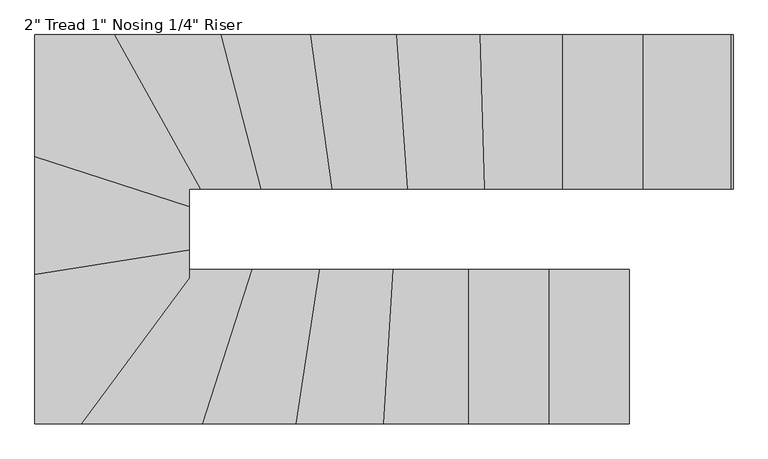
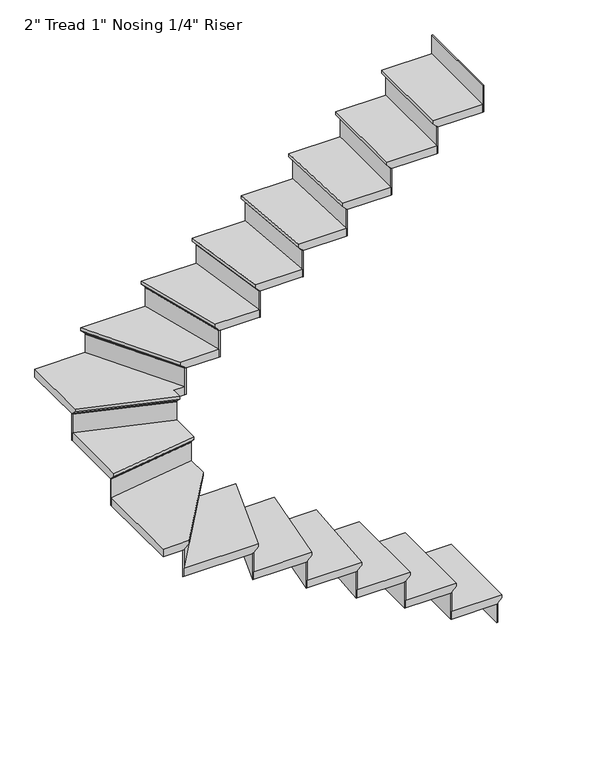
"""IFC4 building model written with IfcOpenShell, lengths in millimetres: stair flight geometry."""

from ifc_helpers import new_model, si_unit, origin, place, context, project, spatial, faceted_brep, source, transform, mapped, element, save


def stair_flight_959e1ed9(model_context):
    return source(origin(), model_context, "Body", "Brep", [
        faceted_brep([(-264.8831579, 264.4433073, 3350.6833333), (-264.8831579, 264.4433073, 3369.7333333), (-264.8831579, -271.8029286, 3369.7333333), (-264.8831579, -271.8029286, 3350.6833333), (-290.2831579, 264.4433073, 3325.2833333), (-290.2831579, -271.8029286, 3325.2833333), (-569.6831579, 264.4433073, 3369.7333333), (-569.6831579, -271.8029286, 3369.7333333), (-290.2831579, -271.8029286, 3318.9333333), (-569.6831579, -271.8029286, 3318.9333333), (-569.6831579, 264.4433073, 3318.9333333), (-290.2831579, 264.4433073, 3318.9333333)], [[[0, 1, 2, 3]], [[4, 0, 3, 5]], [[2, 1, 6, 7]], [[8, 9, 10, 11]], [[2, 7, 9, 8, 5, 3]], [[8, 11, 4, 5]], [[6, 1, 0, 4, 11, 10]], [[7, 6, 10, 9]]]),
        faceted_brep([(-290.2831579, 264.4433073, 3318.9333333), (-290.2831579, 264.4433073, 3200.4), (-296.6331579, 264.4433073, 3200.4), (-296.6331579, 264.4433073, 3318.9333333), (-290.2831579, -271.8029286, 3318.9333333), (-296.6331579, -271.8029286, 3318.9333333), (-296.6331579, -271.8029286, 3200.4), (-290.2831579, -271.8029286, 3200.4)], [[[0, 1, 2, 3]], [[4, 5, 6, 7]], [[1, 0, 4, 7]], [[2, 1, 7, 6]], [[3, 2, 6, 5]], [[0, 3, 5, 4]]]),
        faceted_brep([(-569.6831579, 264.4433073, 3488.2666667), (-569.6831579, 264.4433073, 3318.9333333), (-576.0331579, 264.4433073, 3318.9333333), (-576.0331579, 264.4433073, 3488.2666667), (-569.6831579, -271.8029286, 3488.2666667), (-576.0331579, -271.8029286, 3488.2666667), (-576.0331579, -271.8029286, 3318.9333333), (-569.6831579, -271.8029286, 3318.9333333)], [[[0, 1, 2, 3]], [[4, 5, 6, 7]], [[1, 0, 4, 7]], [[2, 1, 7, 6]], [[3, 2, 6, 5]], [[0, 3, 5, 4]]]),
        faceted_brep([(-544.2831579, -271.8029286, 3539.0666667), (-544.2831579, 264.4433073, 3539.0666667), (-849.0831579, 264.4433073, 3539.0666667), (-849.0831579, -271.8029286, 3539.0666667), (-569.6831579, -271.8029286, 3488.2666667), (-849.0831579, -271.8029286, 3488.2666667), (-849.0831579, 264.4433073, 3488.2666667), (-569.6831579, 264.4433073, 3488.2666667), (-569.6831579, -271.8029286, 3494.6166667), (-544.2831579, -271.8029286, 3520.0166667), (-569.6831579, 264.4433073, 3494.6166667), (-544.2831579, 264.4433073, 3520.0166667)], [[[0, 1, 2, 3]], [[4, 5, 6, 7]], [[0, 3, 5, 4, 8, 9]], [[4, 7, 10, 8]], [[2, 1, 11, 10, 7, 6]], [[3, 2, 6, 5]], [[11, 1, 0, 9]], [[10, 11, 9, 8]]]),
        faceted_brep([(-849.0831579, 264.4433073, 3657.6), (-849.0831579, 264.4433073, 3488.2666667), (-855.4331579, 264.4433073, 3488.2666667), (-855.4331579, 264.4433073, 3657.6), (-849.0831579, -271.8029286, 3657.6), (-855.4331579, -271.8029286, 3657.6), (-855.4331579, -271.8029286, 3488.2666667), (-849.0831579, -271.8029286, 3488.2666667)], [[[0, 1, 2, 3]], [[4, 5, 6, 7]], [[1, 0, 4, 7]], [[2, 1, 7, 6]], [[3, 2, 6, 5]], [[0, 3, 5, 4]]]),
        faceted_brep([(-823.6831579, -271.8029286, 3708.4), (-823.6831579, 264.4433073, 3708.4), (-1112.6009003, 264.4433073, 3708.4), (-1144.4549627, -271.8029286, 3708.4), (-849.0831579, -271.8029286, 3657.6), (-1144.4549627, -271.8029286, 3657.6), (-1112.6009003, 264.4433073, 3657.6), (-849.0831579, 264.4433073, 3657.6), (-849.0831579, -271.8029286, 3663.95), (-823.6831579, -271.8029286, 3689.35), (-849.0831579, 264.4433073, 3663.95), (-823.6831579, 264.4433073, 3689.35)], [[[0, 1, 2, 3]], [[4, 5, 6, 7]], [[0, 3, 5, 4, 8, 9]], [[4, 7, 10, 8]], [[2, 1, 11, 10, 7, 6]], [[3, 2, 6, 5]], [[11, 1, 0, 9]], [[10, 11, 9, 8]]]),
        faceted_brep([(-1112.6009003, 264.4433073, 3826.9333333), (-1112.6009003, 264.4433073, 3657.6), (-1118.9620938, 264.4433073, 3657.6), (-1118.9620938, 264.4433073, 3826.9333333), (-1144.4549627, -271.8029286, 3826.9333333), (-1150.8161561, -271.8029286, 3826.9333333), (-1150.8161561, -271.8029286, 3657.6), (-1144.4549627, -271.8029286, 3657.6)], [[[0, 1, 2, 3]], [[4, 5, 6, 7]], [[1, 0, 4, 7]], [[2, 1, 7, 6]], [[3, 2, 6, 5]], [[0, 3, 5, 4]]]),
        faceted_brep([(-1119.0101891, -271.8029286, 3877.7333333), (-1087.1561267, 264.4433073, 3877.7333333), (-1367.1376579, 264.4433073, 3877.7333333), (-1449.2203373, -271.8029286, 3877.7333333), (-1144.4549627, -271.8029286, 3826.9333333), (-1449.2203373, -271.8029286, 3826.9333333), (-1367.1376579, 264.4433073, 3826.9333333), (-1112.6009003, 264.4433073, 3826.9333333), (-1144.4549627, -271.8029286, 3833.2833333), (-1119.0101891, -271.8029286, 3858.6833333), (-1112.6009003, 264.4433073, 3833.2833333), (-1087.1561267, 264.4433073, 3858.6833333)], [[[0, 1, 2, 3]], [[4, 5, 6, 7]], [[0, 3, 5, 4, 8, 9]], [[4, 7, 10, 8]], [[2, 1, 11, 10, 7, 6]], [[3, 2, 6, 5]], [[11, 1, 0, 9]], [[10, 11, 9, 8]]]),
        faceted_brep([(-1367.1376579, 264.4433073, 3996.2666667), (-1367.1376579, 264.4433073, 3826.9333333), (-1373.5616178, 264.4433073, 3826.9333333), (-1373.5616178, 264.4433073, 3996.2666667), (-1449.2203373, -271.8029286, 3996.2666667), (-1455.6442972, -271.8029286, 3996.2666667), (-1455.6442972, -271.8029286, 3826.9333333), (-1449.2203373, -271.8029286, 3826.9333333)], [[[0, 1, 2, 3]], [[4, 5, 6, 7]], [[1, 0, 4, 7]], [[2, 1, 7, 6]], [[3, 2, 6, 5]], [[0, 3, 5, 4]]]),
        faceted_brep([(-1423.5244976, -271.8029286, 4047.0666667), (-1341.4418182, 264.4433073, 4047.0666667), (-1602.0584075, 264.4433073, 4047.0666667), (-1775.0869242, -271.8029286, 4047.0666667), (-1449.2203373, -271.8029286, 3996.2666667), (-1775.0869242, -271.8029286, 3996.2666667), (-1602.0584075, 264.4433073, 3996.2666667), (-1367.1376579, 264.4433073, 3996.2666667), (-1449.2203373, -271.8029286, 4002.6166667), (-1423.5244976, -271.8029286, 4028.0166667), (-1367.1376579, 264.4433073, 4002.6166667), (-1341.4418182, 264.4433073, 4028.0166667)], [[[0, 1, 2, 3]], [[4, 5, 6, 7]], [[0, 3, 5, 4, 8, 9]], [[4, 7, 10, 8]], [[2, 1, 11, 10, 7, 6]], [[3, 2, 6, 5]], [[11, 1, 0, 9]], [[10, 11, 9, 8]]]),
        faceted_brep([(-1602.0584075, 264.4433073, 4165.6), (-1602.0584075, 264.4433073, 3996.2666667), (-1608.7307845, 264.4433073, 3996.2666667), (-1608.7307845, 264.4433073, 4165.6), (-1775.0869242, -271.8029286, 4165.6), (-1781.7593012, -271.8029286, 4165.6), (-1781.7593012, -271.8029286, 3996.2666667), (-1775.0869242, -271.8029286, 3996.2666667)], [[[0, 1, 2, 3]], [[4, 5, 6, 7]], [[1, 0, 4, 7]], [[2, 1, 7, 6]], [[3, 2, 6, 5]], [[0, 3, 5, 4]]]),
        faceted_brep([(-1748.3974163, -271.8029286, 4216.4), (-1575.3688995, 264.4433073, 4216.4), (-1792.6148498, 264.4433073, 4216.4), (-1792.6148498, 277.721026, 4216.4), (-2200.2950016, -271.8029286, 4216.4), (-1775.0869242, -271.8029286, 4165.6), (-2200.2950016, -271.8029286, 4165.6), (-1792.6148498, 277.721026, 4165.6), (-1792.6148498, 264.4433073, 4165.6), (-1602.0584075, 264.4433073, 4165.6), (-1775.0869242, -271.8029286, 4171.95), (-1748.3974163, -271.8029286, 4197.35), (-1602.0584075, 264.4433073, 4171.95), (-1575.3688995, 264.4433073, 4197.35)], [[[0, 1, 2, 3, 4]], [[5, 6, 7, 8, 9]], [[0, 4, 6, 5, 10, 11]], [[5, 9, 12, 10]], [[2, 1, 13, 12, 9, 8]], [[4, 3, 7, 6]], [[13, 1, 0, 11]], [[12, 13, 11, 10]], [[3, 2, 8, 7]]]),
        faceted_brep([(-1792.6148498, 277.721026, 4334.9333333), (-1792.6148498, 277.721026, 4165.6), (-1792.6148498, 288.3786511, 4165.6), (-1792.6148498, 288.3786511, 4334.9333333), (-2200.2950016, -271.8029286, 4334.9333333), (-2208.2016673, -271.8029286, 4334.9333333), (-2208.2016673, -271.8029286, 4165.6), (-2200.2950016, -271.8029286, 4165.6)], [[[0, 1, 2, 3]], [[4, 5, 6, 7]], [[1, 0, 4, 7]], [[2, 1, 7, 6]], [[3, 2, 6, 5]], [[0, 3, 5, 4]]]),
        faceted_brep([(-2328.8610857, 272.9225747, 4385.7333333), (-2328.8610857, -271.8029286, 4385.7333333), (-2168.6683387, -271.8029286, 4385.7333333), (-1792.6148498, 235.0905257, 4385.7333333), (-1792.6148498, 358.7948785, 4385.7333333), (-2328.8610857, -271.8029286, 4334.9333333), (-2328.8610857, 272.9225747, 4334.9333333), (-1792.6148498, 358.7948785, 4334.9333333), (-1792.6148498, 277.721026, 4334.9333333), (-2200.2950016, -271.8029286, 4334.9333333), (-2200.2950016, -271.8029286, 4341.2833333), (-2168.6683387, -271.8029286, 4366.6833333), (-1792.6148498, 277.721026, 4341.2833333), (-1792.6148498, 235.0905257, 4366.6833333)], [[[0, 1, 2, 3, 4]], [[5, 6, 7, 8, 9]], [[1, 0, 6, 5]], [[2, 1, 5, 9, 10, 11]], [[9, 8, 12, 10]], [[4, 3, 13, 12, 8, 7]], [[0, 4, 7, 6]], [[13, 3, 2, 11]], [[12, 13, 11, 10]]]),
        faceted_brep([(-1792.6148498, 358.7948785, 4504.2666667), (-1792.6148498, 358.7948785, 4334.9333333), (-1792.6148498, 365.2257813, 4334.9333333), (-1792.6148498, 365.2257813, 4504.2666667), (-2328.8610857, 272.9225747, 4504.2666667), (-2328.8610857, 279.3534775, 4504.2666667), (-2328.8610857, 279.3534775, 4334.9333333), (-2328.8610857, 272.9225747, 4334.9333333)], [[[0, 1, 2, 3]], [[4, 5, 6, 7]], [[1, 0, 4, 7]], [[2, 1, 7, 6]], [[3, 2, 6, 5]], [[0, 3, 5, 4]]]),
        faceted_brep([(-2328.8610857, 247.1989634, 4555.0666667), (-1792.6148498, 333.0712672, 4555.0666667), (-1792.6148498, 510.0383883, 4555.0666667), (-2328.8610857, 683.2061106, 4555.0666667), (-2328.8610857, 272.9225747, 4504.2666667), (-2328.8610857, 683.2061106, 4504.2666667), (-1792.6148498, 510.0383883, 4504.2666667), (-1792.6148498, 358.7948785, 4504.2666667), (-2328.8610857, 272.9225747, 4510.6166667), (-2328.8610857, 247.1989634, 4536.0166667), (-1792.6148498, 358.7948785, 4510.6166667), (-1792.6148498, 333.0712672, 4536.0166667)], [[[0, 1, 2, 3]], [[4, 5, 6, 7]], [[0, 3, 5, 4, 8, 9]], [[4, 7, 10, 8]], [[3, 2, 6, 5]], [[11, 1, 0, 9]], [[10, 11, 9, 8]], [[2, 1, 11, 10, 7, 6]]]),
        faceted_brep([(-1792.6148498, 510.0383883, 4673.6), (-1792.6148498, 510.0383883, 4504.2666667), (-1792.6148498, 516.7112716, 4504.2666667), (-1792.6148498, 516.7112716, 4673.6), (-2328.8610857, 683.2061106, 4673.6), (-2328.8610857, 689.878994, 4673.6), (-2328.8610857, 689.878994, 4504.2666667), (-2328.8610857, 683.2061106, 4504.2666667)], [[[0, 1, 2, 3]], [[4, 5, 6, 7]], [[1, 0, 4, 7]], [[2, 1, 7, 6]], [[3, 2, 6, 5]], [[0, 3, 5, 4]]]),
        faceted_brep([(-2021.9568272, 1080.0895433, 4724.4), (-2328.8610857, 1080.0895433, 4724.4), (-2328.8610857, 656.5145772, 4724.4), (-1792.6148498, 483.3468548, 4724.4), (-1792.6148498, 543.8433073, 4724.4), (-1724.5287393, 543.8433073, 4724.4), (-2328.8610857, 1080.0895433, 4673.6), (-2021.9568272, 1080.0895433, 4673.6), (-1724.5287393, 543.8433073, 4673.6), (-1792.6148498, 543.8433073, 4673.6), (-1792.6148498, 510.0383883, 4673.6), (-2328.8610857, 683.2061106, 4673.6), (-1792.6148498, 510.0383883, 4679.95), (-2328.8610857, 683.2061106, 4679.95), (-1792.6148498, 483.3468548, 4705.35), (-2328.8610857, 656.5145772, 4705.35)], [[[0, 1, 2, 3, 4, 5]], [[6, 7, 8, 9, 10, 11]], [[1, 0, 7, 6]], [[11, 10, 12, 13]], [[4, 3, 14, 12, 10, 9]], [[0, 5, 8, 7]], [[14, 3, 2, 15]], [[12, 14, 15, 13]], [[2, 1, 6, 11, 13, 15]], [[5, 4, 9, 8]]]),
        faceted_brep([(-1724.5287393, 543.8433073, 4842.9333333), (-1724.5287393, 543.8433073, 4673.6), (-1717.2673962, 543.8433073, 4673.6), (-1717.2673962, 543.8433073, 4842.9333333), (-2021.9568272, 1080.0895433, 4842.9333333), (-2014.6954841, 1080.0895433, 4842.9333333), (-2014.6954841, 1080.0895433, 4673.6), (-2021.9568272, 1080.0895433, 4673.6)], [[[0, 1, 2, 3]], [[4, 5, 6, 7]], [[1, 0, 4, 7]], [[2, 1, 7, 6]], [[3, 2, 6, 5]], [[0, 3, 5, 4]]]),
        faceted_brep([(-2051.0021996, 1080.0895433, 4893.7333333), (-1753.5741117, 543.8433073, 4893.7333333), (-1517.487325, 543.8433073, 4893.7333333), (-1656.0375972, 1080.0895433, 4893.7333333), (-2021.9568272, 1080.0895433, 4842.9333333), (-1656.0375972, 1080.0895433, 4842.9333333), (-1517.487325, 543.8433073, 4842.9333333), (-1724.5287393, 543.8433073, 4842.9333333), (-2021.9568272, 1080.0895433, 4849.2833333), (-2051.0021996, 1080.0895433, 4874.6833333), (-1724.5287393, 543.8433073, 4849.2833333), (-1753.5741117, 543.8433073, 4874.6833333)], [[[0, 1, 2, 3]], [[4, 5, 6, 7]], [[0, 3, 5, 4, 8, 9]], [[4, 7, 10, 8]], [[2, 1, 11, 10, 7, 6]], [[3, 2, 6, 5]], [[11, 1, 0, 9]], [[10, 11, 9, 8]]]),
        faceted_brep([(-1517.487325, 543.8433073, 5012.2666667), (-1517.487325, 543.8433073, 4842.9333333), (-1510.9288005, 543.8433073, 4842.9333333), (-1510.9288005, 543.8433073, 5012.2666667), (-1656.0375972, 1080.0895433, 5012.2666667), (-1649.4790727, 1080.0895433, 5012.2666667), (-1649.4790727, 1080.0895433, 4842.9333333), (-1656.0375972, 1080.0895433, 4842.9333333)], [[[0, 1, 2, 3]], [[4, 5, 6, 7]], [[1, 0, 4, 7]], [[2, 1, 7, 6]], [[3, 2, 6, 5]], [[0, 3, 5, 4]]]),
        faceted_brep([(-1682.2716952, 1080.0895433, 5063.0666667), (-1543.721423, 543.8433073, 5063.0666667), (-1271.2041837, 543.8433073, 5063.0666667), (-1344.713853, 1080.0895433, 5063.0666667), (-1656.0375972, 1080.0895433, 5012.2666667), (-1344.713853, 1080.0895433, 5012.2666667), (-1271.2041837, 543.8433073, 5012.2666667), (-1517.487325, 543.8433073, 5012.2666667), (-1656.0375972, 1080.0895433, 5018.6166667), (-1682.2716952, 1080.0895433, 5044.0166667), (-1517.487325, 543.8433073, 5018.6166667), (-1543.721423, 543.8433073, 5044.0166667)], [[[0, 1, 2, 3]], [[4, 5, 6, 7]], [[0, 3, 5, 4, 8, 9]], [[4, 7, 10, 8]], [[2, 1, 11, 10, 7, 6]], [[3, 2, 6, 5]], [[11, 1, 0, 9]], [[10, 11, 9, 8]]]),
        faceted_brep([(-1271.2041837, 543.8433073, 5181.6), (-1271.2041837, 543.8433073, 5012.2666667), (-1264.7947985, 543.8433073, 5012.2666667), (-1264.7947985, 543.8433073, 5181.6), (-1344.713853, 1080.0895433, 5181.6), (-1338.3044678, 1080.0895433, 5181.6), (-1338.3044678, 1080.0895433, 5012.2666667), (-1344.713853, 1080.0895433, 5012.2666667)], [[[0, 1, 2, 3]], [[4, 5, 6, 7]], [[1, 0, 4, 7]], [[2, 1, 7, 6]], [[3, 2, 6, 5]], [[0, 3, 5, 4]]]),
        faceted_brep([(-1370.3513937, 1080.0895433, 5232.4), (-1296.8417245, 543.8433073, 5232.4), (-1009.7763573, 543.8433073, 5232.4), (-1047.6899509, 1080.0895433, 5232.4), (-1344.713853, 1080.0895433, 5181.6), (-1047.6899509, 1080.0895433, 5181.6), (-1009.7763573, 543.8433073, 5181.6), (-1271.2041837, 543.8433073, 5181.6), (-1344.713853, 1080.0895433, 5187.95), (-1370.3513937, 1080.0895433, 5213.35), (-1271.2041837, 543.8433073, 5187.95), (-1296.8417245, 543.8433073, 5213.35)], [[[0, 1, 2, 3]], [[4, 5, 6, 7]], [[0, 3, 5, 4, 8, 9]], [[4, 7, 10, 8]], [[2, 1, 11, 10, 7, 6]], [[3, 2, 6, 5]], [[11, 1, 0, 9]], [[10, 11, 9, 8]]]),
        faceted_brep([(-1009.7763573, 543.8433073, 5350.9333333), (-1009.7763573, 543.8433073, 5181.6), (-1003.4105061, 543.8433073, 5181.6), (-1003.4105061, 543.8433073, 5350.9333333), (-1047.6899509, 1080.0895433, 5350.9333333), (-1041.3240997, 1080.0895433, 5350.9333333), (-1041.3240997, 1080.0895433, 5181.6), (-1047.6899509, 1080.0895433, 5181.6)], [[[0, 1, 2, 3]], [[4, 5, 6, 7]], [[1, 0, 4, 7]], [[2, 1, 7, 6]], [[3, 2, 6, 5]], [[0, 3, 5, 4]]]),
        faceted_brep([(-1073.1533559, 1080.0895433, 5401.7333333), (-1035.2397623, 543.8433073, 5401.7333333), (-741.6570892, 543.8433073, 5401.7333333), (-757.1149275, 1080.0895433, 5401.7333333), (-1047.6899509, 1080.0895433, 5350.9333333), (-757.1149275, 1080.0895433, 5350.9333333), (-741.6570892, 543.8433073, 5350.9333333), (-1009.7763573, 543.8433073, 5350.9333333), (-1047.6899509, 1080.0895433, 5357.2833333), (-1073.1533559, 1080.0895433, 5382.6833333), (-1009.7763573, 543.8433073, 5357.2833333), (-1035.2397623, 543.8433073, 5382.6833333)], [[[0, 1, 2, 3]], [[4, 5, 6, 7]], [[0, 3, 5, 4, 8, 9]], [[4, 7, 10, 8]], [[2, 1, 11, 10, 7, 6]], [[3, 2, 6, 5]], [[11, 1, 0, 9]], [[10, 11, 9, 8]]]),
        faceted_brep([(-741.6570892, 543.8433073, 5520.2666667), (-741.6570892, 543.8433073, 5350.9333333), (-735.3044516, 543.8433073, 5350.9333333), (-735.3044516, 543.8433073, 5520.2666667), (-757.1149275, 1080.0895433, 5520.2666667), (-750.7622898, 1080.0895433, 5520.2666667), (-750.7622898, 1080.0895433, 5350.9333333), (-757.1149275, 1080.0895433, 5350.9333333)], [[[0, 1, 2, 3]], [[4, 5, 6, 7]], [[1, 0, 4, 7]], [[2, 1, 7, 6]], [[3, 2, 6, 5]], [[0, 3, 5, 4]]]),
        faceted_brep([(-782.5254783, 1080.0895433, 5571.0666667), (-767.06764, 543.8433073, 5571.0666667), (-469.9965591, 543.8433073, 5571.0666667), (-469.9965591, 1080.0895433, 5571.0666667), (-757.1149275, 1080.0895433, 5520.2666667), (-469.9965591, 1080.0895433, 5520.2666667), (-469.9965591, 543.8433073, 5520.2666667), (-741.6570892, 543.8433073, 5520.2666667), (-757.1149275, 1080.0895433, 5526.6166667), (-782.5254783, 1080.0895433, 5552.0166667), (-741.6570892, 543.8433073, 5526.6166667), (-767.06764, 543.8433073, 5552.0166667)], [[[0, 1, 2, 3]], [[4, 5, 6, 7]], [[0, 3, 5, 4, 8, 9]], [[4, 7, 10, 8]], [[2, 1, 11, 10, 7, 6]], [[3, 2, 6, 5]], [[11, 1, 0, 9]], [[10, 11, 9, 8]]]),
        faceted_brep([(-469.9965591, 543.8433073, 5689.6), (-469.9965591, 543.8433073, 5520.2666667), (-463.6465591, 543.8433073, 5520.2666667), (-463.6465591, 543.8433073, 5689.6), (-469.9965591, 1080.0895433, 5689.6), (-463.6465591, 1080.0895433, 5689.6), (-463.6465591, 1080.0895433, 5520.2666667), (-469.9965591, 1080.0895433, 5520.2666667)], [[[0, 1, 2, 3]], [[4, 5, 6, 7]], [[1, 0, 4, 7]], [[2, 1, 7, 6]], [[3, 2, 6, 5]], [[0, 3, 5, 4]]]),
        faceted_brep([(-495.3965591, 1080.0895433, 5740.4), (-495.3965591, 543.8433073, 5740.4), (-190.5965591, 543.8433073, 5740.4), (-190.5965591, 1080.0895433, 5740.4), (-469.9965591, 1080.0895433, 5689.6), (-190.5965591, 1080.0895433, 5689.6), (-190.5965591, 543.8433073, 5689.6), (-469.9965591, 543.8433073, 5689.6), (-469.9965591, 1080.0895433, 5695.95), (-495.3965591, 1080.0895433, 5721.35), (-469.9965591, 543.8433073, 5695.95), (-495.3965591, 543.8433073, 5721.35)], [[[0, 1, 2, 3]], [[4, 5, 6, 7]], [[0, 3, 5, 4, 8, 9]], [[4, 7, 10, 8]], [[2, 1, 11, 10, 7, 6]], [[3, 2, 6, 5]], [[11, 1, 0, 9]], [[10, 11, 9, 8]]]),
        faceted_brep([(-190.5965591, 543.8433073, 5858.9333333), (-190.5965591, 543.8433073, 5689.6), (-184.2465591, 543.8433073, 5689.6), (-184.2465591, 543.8433073, 5858.9333333), (-190.5965591, 1080.0895433, 5858.9333333), (-184.2465591, 1080.0895433, 5858.9333333), (-184.2465591, 1080.0895433, 5689.6), (-190.5965591, 1080.0895433, 5689.6)], [[[0, 1, 2, 3]], [[4, 5, 6, 7]], [[1, 0, 4, 7]], [[2, 1, 7, 6]], [[3, 2, 6, 5]], [[0, 3, 5, 4]]]),
        faceted_brep([(88.8034409, 543.8433073, 6028.2666667), (88.8034409, 543.8433073, 5858.9333333), (95.1534409, 543.8433073, 5858.9333333), (95.1534409, 543.8433073, 6028.2666667), (88.8034409, 1080.0895433, 6028.2666667), (95.1534409, 1080.0895433, 6028.2666667), (95.1534409, 1080.0895433, 5858.9333333), (88.8034409, 1080.0895433, 5858.9333333)], [[[0, 1, 2, 3]], [[4, 5, 6, 7]], [[1, 0, 4, 7]], [[2, 1, 7, 6]], [[3, 2, 6, 5]], [[0, 3, 5, 4]]]),
        faceted_brep([(-215.9965591, 1080.0895433, 5909.7333333), (-215.9965591, 543.8433073, 5909.7333333), (88.8034409, 543.8433073, 5909.7333333), (88.8034409, 1080.0895433, 5909.7333333), (-190.5965591, 1080.0895433, 5858.9333333), (88.8034409, 1080.0895433, 5858.9333333), (88.8034409, 543.8433073, 5858.9333333), (-190.5965591, 543.8433073, 5858.9333333), (-190.5965591, 1080.0895433, 5865.2833333), (-215.9965591, 1080.0895433, 5890.6833333), (-190.5965591, 543.8433073, 5865.2833333), (-215.9965591, 543.8433073, 5890.6833333)], [[[0, 1, 2, 3]], [[4, 5, 6, 7]], [[0, 3, 5, 4, 8, 9]], [[4, 7, 10, 8]], [[2, 1, 11, 10, 7, 6]], [[3, 2, 6, 5]], [[11, 1, 0, 9]], [[10, 11, 9, 8]]]),
    ])


if __name__ == "__main__":
    model = new_model("IFC4")
    model_context = context("Model", 3, world=origin())
    ifc_project = project(units=[si_unit("LENGTHUNIT", "METRE", prefix="MILLI")], contexts=[model_context])
    site = spatial("IfcSite", under=ifc_project)
    building = spatial("IfcBuilding", under=site)
    placement = place(None, origin())
    stair_flight_shape = stair_flight_959e1ed9(model_context)
    element("IfcStairFlight", 1, ObjectType="2\" Tread 1\" Nosing 1/4\" Riser", at=placement, inside=building, context=model_context, shape_type="MappedRepresentation", body=[
        mapped(stair_flight_shape, transform((0.0, 0.0, 0.0), x_axis=(1.0, 0.0, 0.0), y_axis=(0.0, 1.0, 0.0), z_axis=(0.0, 0.0, 1.0))),
    ])
    save(model, "model.ifc")
